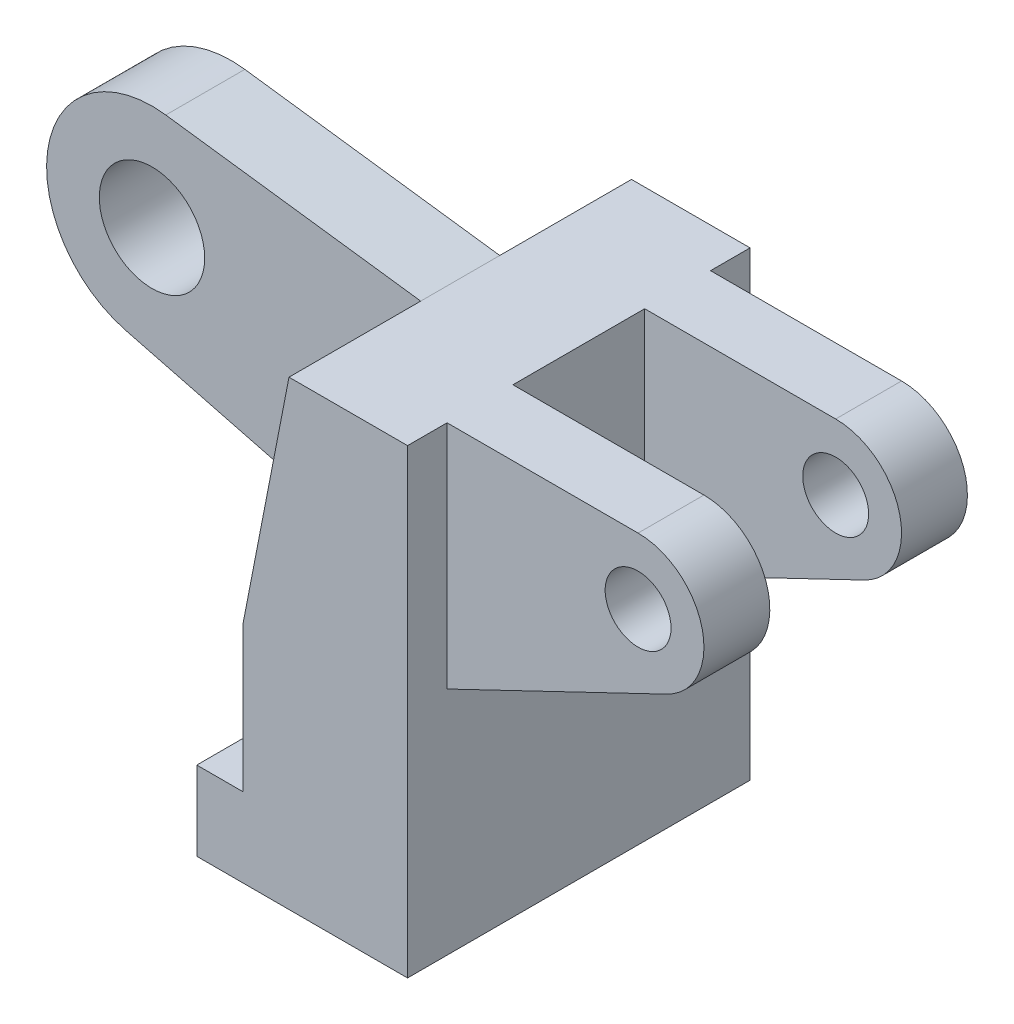
ISO-10303-21;
HEADER;
FILE_DESCRIPTION(('STEP AP214'),'2;1');
FILE_NAME('part.step','',(''),(''),'','','');
FILE_SCHEMA(('AUTOMOTIVE_DESIGN { 1 0 10303 214 1 1 1 1 }'));
ENDSEC;
DATA;
#1=APPLICATION_CONTEXT('core data for automotive mechanical design processes');
#2=APPLICATION_PROTOCOL_DEFINITION('international standard','automotive_design',2000,#1);
#3=PRODUCT_CONTEXT('',#1,'mechanical');
#4=PRODUCT('Part','Part','',(#3));
#5=PRODUCT_RELATED_PRODUCT_CATEGORY('part','',(#4));
#6=PRODUCT_DEFINITION_FORMATION('','',#4);
#7=PRODUCT_DEFINITION_CONTEXT('part definition',#1,'design');
#8=PRODUCT_DEFINITION('design','',#6,#7);
#9=PRODUCT_DEFINITION_SHAPE('','',#8);
#10=(LENGTH_UNIT() NAMED_UNIT(*) SI_UNIT(.MILLI.,.METRE.));
#11=(NAMED_UNIT(*) PLANE_ANGLE_UNIT() SI_UNIT($,.RADIAN.));
#12=(NAMED_UNIT(*) SI_UNIT($,.STERADIAN.) SOLID_ANGLE_UNIT());
#13=UNCERTAINTY_MEASURE_WITH_UNIT(LENGTH_MEASURE(1.E-05),#10,'distance_accuracy_value','');
#14=(GEOMETRIC_REPRESENTATION_CONTEXT(3) GLOBAL_UNCERTAINTY_ASSIGNED_CONTEXT((#13)) GLOBAL_UNIT_ASSIGNED_CONTEXT((#10,
#11,#12)) REPRESENTATION_CONTEXT('',''));
#15=CARTESIAN_POINT('',(0.,0.,0.));
#16=DIRECTION('',(0.,0.,1.));
#17=DIRECTION('',(1.,0.,0.));
#18=AXIS2_PLACEMENT_3D('',#15,#16,#17);
#19=CARTESIAN_POINT('',(7.,34.,0.));
#20=DIRECTION('',(-0.981615389668581,0.190869659102224,0.));
#21=DIRECTION('',(-0.190869659102224,-0.981615389668581,0.));
#22=AXIS2_PLACEMENT_3D('',#19,#20,#21);
#23=PLANE('',#22);
#24=DIRECTION('',(0.,0.,1.));
#25=VECTOR('',#24,1.);
#26=CARTESIAN_POINT('',(7.,34.,0.));
#27=LINE('',#26,#25);
#28=CARTESIAN_POINT('',(7.,34.,0.));
#29=VERTEX_POINT('',#28);
#30=CARTESIAN_POINT('',(7.,34.,20.));
#31=VERTEX_POINT('',#30);
#32=EDGE_CURVE('E206',#29,#31,#27,.T.);
#33=ORIENTED_EDGE('',*,*,#32,.T.);
#34=DIRECTION('',(-0.190869659102224,-0.981615389668581,0.));
#35=VECTOR('',#34,1.);
#36=CARTESIAN_POINT('',(0.374721189591083,-0.0728624535315993,20.));
#37=LINE('',#36,#35);
#38=CARTESIAN_POINT('',(14.,70.,20.));
#39=VERTEX_POINT('',#38);
#40=EDGE_CURVE('E543',#39,#31,#37,.T.);
#41=ORIENTED_EDGE('',*,*,#40,.F.);
#42=DIRECTION('',(0.,0.,1.));
#43=VECTOR('',#42,1.);
#44=CARTESIAN_POINT('',(14.,70.,0.));
#45=LINE('',#44,#43);
#46=CARTESIAN_POINT('',(14.,70.,0.));
#47=VERTEX_POINT('',#46);
#48=EDGE_CURVE('E210',#47,#39,#45,.T.);
#49=ORIENTED_EDGE('',*,*,#48,.F.);
#50=DIRECTION('',(-0.190869659102224,-0.981615389668581,0.));
#51=VECTOR('',#50,1.);
#52=CARTESIAN_POINT('',(7.,34.,0.));
#53=LINE('',#52,#51);
#54=EDGE_CURVE('E258',#47,#29,#53,.T.);
#55=ORIENTED_EDGE('',*,*,#54,.T.);
#56=EDGE_LOOP('',(#33,#41,#49,#55));
#57=FACE_BOUND('',#56,.T.);
#58=ADVANCED_FACE('F41',(#57),#23,.T.);
#59=CARTESIAN_POINT('',(0.,12.,52.));
#60=DIRECTION('',(0.,-1.,0.));
#61=DIRECTION('',(0.,0.,-1.));
#62=AXIS2_PLACEMENT_3D('',#59,#60,#61);
#63=PLANE('',#62);
#64=DIRECTION('',(0.,0.,1.));
#65=VECTOR('',#64,1.);
#66=CARTESIAN_POINT('',(7.,12.,0.));
#67=LINE('',#66,#65);
#68=CARTESIAN_POINT('',(7.,12.,0.));
#69=VERTEX_POINT('',#68);
#70=CARTESIAN_POINT('',(7.,12.,52.));
#71=VERTEX_POINT('',#70);
#72=EDGE_CURVE('E207',#69,#71,#67,.T.);
#73=ORIENTED_EDGE('',*,*,#72,.F.);
#74=DIRECTION('',(-1.,0.,0.));
#75=VECTOR('',#74,1.);
#76=CARTESIAN_POINT('',(0.,12.,0.));
#77=LINE('',#76,#75);
#78=CARTESIAN_POINT('',(0.,12.,0.));
#79=VERTEX_POINT('',#78);
#80=EDGE_CURVE('E224',#69,#79,#77,.T.);
#81=ORIENTED_EDGE('',*,*,#80,.T.);
#82=DIRECTION('',(0.,0.,-1.));
#83=VECTOR('',#82,1.);
#84=CARTESIAN_POINT('',(0.,12.,52.));
#85=LINE('',#84,#83);
#86=CARTESIAN_POINT('',(0.,12.,52.));
#87=VERTEX_POINT('',#86);
#88=EDGE_CURVE('E226',#87,#79,#85,.T.);
#89=ORIENTED_EDGE('',*,*,#88,.F.);
#90=DIRECTION('',(-1.,0.,0.));
#91=VECTOR('',#90,1.);
#92=CARTESIAN_POINT('',(0.,12.,52.));
#93=LINE('',#92,#91);
#94=EDGE_CURVE('E227',#71,#87,#93,.T.);
#95=ORIENTED_EDGE('',*,*,#94,.F.);
#96=EDGE_LOOP('',(#73,#81,#89,#95));
#97=FACE_BOUND('',#96,.T.);
#98=ADVANCED_FACE('F389',(#97),#63,.F.);
#99=CARTESIAN_POINT('',(0.,0.,52.));
#100=DIRECTION('',(1.,0.,0.));
#101=DIRECTION('',(0.,0.,-1.));
#102=AXIS2_PLACEMENT_3D('',#99,#100,#101);
#103=PLANE('',#102);
#104=DIRECTION('',(0.,-1.,0.));
#105=VECTOR('',#104,1.);
#106=CARTESIAN_POINT('',(0.,0.,0.));
#107=LINE('',#106,#105);
#108=CARTESIAN_POINT('',(0.,0.,0.));
#109=VERTEX_POINT('',#108);
#110=EDGE_CURVE('E232',#79,#109,#107,.T.);
#111=ORIENTED_EDGE('',*,*,#110,.T.);
#112=DIRECTION('',(0.,0.,-1.));
#113=VECTOR('',#112,1.);
#114=CARTESIAN_POINT('',(0.,0.,52.));
#115=LINE('',#114,#113);
#116=CARTESIAN_POINT('',(0.,0.,52.));
#117=VERTEX_POINT('',#116);
#118=EDGE_CURVE('E11',#117,#109,#115,.T.);
#119=ORIENTED_EDGE('',*,*,#118,.F.);
#120=DIRECTION('',(0.,-1.,0.));
#121=VECTOR('',#120,1.);
#122=CARTESIAN_POINT('',(0.,0.,52.));
#123=LINE('',#122,#121);
#124=EDGE_CURVE('E218',#87,#117,#123,.T.);
#125=ORIENTED_EDGE('',*,*,#124,.F.);
#126=ORIENTED_EDGE('',*,*,#88,.T.);
#127=EDGE_LOOP('',(#111,#119,#125,#126));
#128=FACE_BOUND('',#127,.T.);
#129=ADVANCED_FACE('F43',(#128),#103,.F.);
#130=CARTESIAN_POINT('',(0.,0.,52.));
#131=DIRECTION('',(0.,1.,0.));
#132=DIRECTION('',(0.,0.,1.));
#133=AXIS2_PLACEMENT_3D('',#130,#131,#132);
#134=PLANE('',#133);
#135=DIRECTION('',(1.,0.,0.));
#136=VECTOR('',#135,1.);
#137=CARTESIAN_POINT('',(0.,0.,0.));
#138=LINE('',#137,#136);
#139=CARTESIAN_POINT('',(32.,0.,0.));
#140=VERTEX_POINT('',#139);
#141=EDGE_CURVE('E231',#109,#140,#138,.T.);
#142=ORIENTED_EDGE('',*,*,#141,.T.);
#143=DIRECTION('',(0.,0.,-1.));
#144=VECTOR('',#143,1.);
#145=CARTESIAN_POINT('',(32.,0.,52.));
#146=LINE('',#145,#144);
#147=CARTESIAN_POINT('',(32.,0.,52.));
#148=VERTEX_POINT('',#147);
#149=EDGE_CURVE('E47',#148,#140,#146,.T.);
#150=ORIENTED_EDGE('',*,*,#149,.F.);
#151=DIRECTION('',(1.,0.,0.));
#152=VECTOR('',#151,1.);
#153=CARTESIAN_POINT('',(0.,0.,52.));
#154=LINE('',#153,#152);
#155=EDGE_CURVE('E225',#117,#148,#154,.T.);
#156=ORIENTED_EDGE('',*,*,#155,.F.);
#157=ORIENTED_EDGE('',*,*,#118,.T.);
#158=EDGE_LOOP('',(#142,#150,#156,#157));
#159=FACE_BOUND('',#158,.T.);
#160=ADVANCED_FACE('F426',(#159),#134,.F.);
#161=CARTESIAN_POINT('',(32.,12.,52.));
#162=DIRECTION('',(-1.,0.,0.));
#163=DIRECTION('',(0.,0.,1.));
#164=AXIS2_PLACEMENT_3D('',#161,#162,#163);
#165=PLANE('',#164);
#166=DIRECTION('',(0.,0.,1.));
#167=VECTOR('',#166,1.);
#168=CARTESIAN_POINT('',(32.,70.,0.));
#169=LINE('',#168,#167);
#170=CARTESIAN_POINT('',(32.,70.,16.));
#171=VERTEX_POINT('',#170);
#172=CARTESIAN_POINT('',(32.,70.,36.));
#173=VERTEX_POINT('',#172);
#174=EDGE_CURVE('E220',#171,#173,#169,.T.);
#175=ORIENTED_EDGE('',*,*,#174,.T.);
#176=DIRECTION('',(0.,-1.,0.));
#177=VECTOR('',#176,1.);
#178=CARTESIAN_POINT('',(32.,70.,36.));
#179=LINE('',#178,#177);
#180=CARTESIAN_POINT('',(32.,35.,36.));
#181=VERTEX_POINT('',#180);
#182=EDGE_CURVE('E65',#173,#181,#179,.T.);
#183=ORIENTED_EDGE('',*,*,#182,.T.);
#184=DIRECTION('',(0.,0.,1.));
#185=VECTOR('',#184,1.);
#186=CARTESIAN_POINT('',(32.,35.,36.));
#187=LINE('',#186,#185);
#188=CARTESIAN_POINT('',(32.,35.,46.));
#189=VERTEX_POINT('',#188);
#190=EDGE_CURVE('E301',#181,#189,#187,.T.);
#191=ORIENTED_EDGE('',*,*,#190,.T.);
#192=DIRECTION('',(0.,-1.,0.));
#193=VECTOR('',#192,1.);
#194=CARTESIAN_POINT('',(32.,70.,46.));
#195=LINE('',#194,#193);
#196=CARTESIAN_POINT('',(32.,70.,46.));
#197=VERTEX_POINT('',#196);
#198=EDGE_CURVE('E288',#197,#189,#195,.T.);
#199=ORIENTED_EDGE('',*,*,#198,.F.);
#200=CARTESIAN_POINT('',(32.,70.,52.));
#201=VERTEX_POINT('',#200);
#202=EDGE_CURVE('E217',#197,#201,#169,.T.);
#203=ORIENTED_EDGE('',*,*,#202,.T.);
#204=DIRECTION('',(0.,1.,0.));
#205=VECTOR('',#204,1.);
#206=CARTESIAN_POINT('',(32.,12.,52.));
#207=LINE('',#206,#205);
#208=EDGE_CURVE('E223',#148,#201,#207,.T.);
#209=ORIENTED_EDGE('',*,*,#208,.F.);
#210=ORIENTED_EDGE('',*,*,#149,.T.);
#211=DIRECTION('',(0.,1.,0.));
#212=VECTOR('',#211,1.);
#213=CARTESIAN_POINT('',(32.,12.,0.));
#214=LINE('',#213,#212);
#215=CARTESIAN_POINT('',(32.,70.,0.));
#216=VERTEX_POINT('',#215);
#217=EDGE_CURVE('E237',#140,#216,#214,.T.);
#218=ORIENTED_EDGE('',*,*,#217,.T.);
#219=CARTESIAN_POINT('',(32.,70.,6.));
#220=VERTEX_POINT('',#219);
#221=EDGE_CURVE('E214',#216,#220,#169,.T.);
#222=ORIENTED_EDGE('',*,*,#221,.T.);
#223=DIRECTION('',(0.,-1.,0.));
#224=VECTOR('',#223,1.);
#225=CARTESIAN_POINT('',(32.,70.,6.));
#226=LINE('',#225,#224);
#227=CARTESIAN_POINT('',(32.,35.,6.));
#228=VERTEX_POINT('',#227);
#229=EDGE_CURVE('E322',#220,#228,#226,.T.);
#230=ORIENTED_EDGE('',*,*,#229,.T.);
#231=DIRECTION('',(0.,0.,-1.));
#232=VECTOR('',#231,1.);
#233=CARTESIAN_POINT('',(32.,35.,16.));
#234=LINE('',#233,#232);
#235=CARTESIAN_POINT('',(32.,35.,16.));
#236=VERTEX_POINT('',#235);
#237=EDGE_CURVE('E263',#236,#228,#234,.T.);
#238=ORIENTED_EDGE('',*,*,#237,.F.);
#239=DIRECTION('',(0.,-1.,0.));
#240=VECTOR('',#239,1.);
#241=CARTESIAN_POINT('',(32.,70.,16.));
#242=LINE('',#241,#240);
#243=EDGE_CURVE('E330',#171,#236,#242,.T.);
#244=ORIENTED_EDGE('',*,*,#243,.F.);
#245=EDGE_LOOP('',(#175,#183,#191,#199,#203,#209,#210,#218,#222,#230,#238,#244));
#246=FACE_BOUND('',#245,.T.);
#247=ADVANCED_FACE('F245',(#246),#165,.F.);
#248=CARTESIAN_POINT('',(0.,0.,52.));
#249=DIRECTION('',(0.,0.,-1.));
#250=DIRECTION('',(-1.,0.,0.));
#251=AXIS2_PLACEMENT_3D('',#248,#249,#250);
#252=PLANE('',#251);
#253=ORIENTED_EDGE('',*,*,#124,.T.);
#254=ORIENTED_EDGE('',*,*,#155,.T.);
#255=ORIENTED_EDGE('',*,*,#208,.T.);
#256=DIRECTION('',(-1.,0.,0.));
#257=VECTOR('',#256,1.);
#258=CARTESIAN_POINT('',(32.,70.,52.));
#259=LINE('',#258,#257);
#260=CARTESIAN_POINT('',(14.,70.,52.));
#261=VERTEX_POINT('',#260);
#262=EDGE_CURVE('E268',#201,#261,#259,.T.);
#263=ORIENTED_EDGE('',*,*,#262,.T.);
#264=DIRECTION('',(-0.190869659102224,-0.981615389668581,0.));
#265=VECTOR('',#264,1.);
#266=CARTESIAN_POINT('',(7.,34.,52.));
#267=LINE('',#266,#265);
#268=CARTESIAN_POINT('',(7.,34.,52.));
#269=VERTEX_POINT('',#268);
#270=EDGE_CURVE('E261',#261,#269,#267,.T.);
#271=ORIENTED_EDGE('',*,*,#270,.T.);
#272=DIRECTION('',(0.,-1.,0.));
#273=VECTOR('',#272,1.);
#274=CARTESIAN_POINT('',(7.,12.,52.));
#275=LINE('',#274,#273);
#276=EDGE_CURVE('E202',#269,#71,#275,.T.);
#277=ORIENTED_EDGE('',*,*,#276,.T.);
#278=ORIENTED_EDGE('',*,*,#94,.T.);
#279=EDGE_LOOP('',(#253,#254,#255,#263,#271,#277,#278));
#280=FACE_BOUND('',#279,.T.);
#281=ADVANCED_FACE('F275',(#280),#252,.F.);
#282=CARTESIAN_POINT('',(0.,0.,0.));
#283=DIRECTION('',(0.,0.,-1.));
#284=DIRECTION('',(-1.,0.,0.));
#285=AXIS2_PLACEMENT_3D('',#282,#283,#284);
#286=PLANE('',#285);
#287=ORIENTED_EDGE('',*,*,#110,.F.);
#288=ORIENTED_EDGE('',*,*,#80,.F.);
#289=DIRECTION('',(0.,-1.,0.));
#290=VECTOR('',#289,1.);
#291=CARTESIAN_POINT('',(7.,12.,0.));
#292=LINE('',#291,#290);
#293=EDGE_CURVE('E259',#29,#69,#292,.T.);
#294=ORIENTED_EDGE('',*,*,#293,.F.);
#295=ORIENTED_EDGE('',*,*,#54,.F.);
#296=DIRECTION('',(-1.,0.,0.));
#297=VECTOR('',#296,1.);
#298=CARTESIAN_POINT('',(32.,70.,0.));
#299=LINE('',#298,#297);
#300=EDGE_CURVE('E251',#216,#47,#299,.T.);
#301=ORIENTED_EDGE('',*,*,#300,.F.);
#302=ORIENTED_EDGE('',*,*,#217,.F.);
#303=ORIENTED_EDGE('',*,*,#141,.F.);
#304=EDGE_LOOP('',(#287,#288,#294,#295,#301,#302,#303));
#305=FACE_BOUND('',#304,.T.);
#306=ADVANCED_FACE('F248',(#305),#286,.T.);
#307=CARTESIAN_POINT('',(7.,12.,0.));
#308=DIRECTION('',(-1.,0.,0.));
#309=DIRECTION('',(0.,0.,1.));
#310=AXIS2_PLACEMENT_3D('',#307,#308,#309);
#311=PLANE('',#310);
#312=ORIENTED_EDGE('',*,*,#276,.F.);
#313=CARTESIAN_POINT('',(7.,34.,32.));
#314=VERTEX_POINT('',#313);
#315=EDGE_CURVE('E193',#314,#269,#27,.T.);
#316=ORIENTED_EDGE('',*,*,#315,.F.);
#317=DIRECTION('',(0.,0.,-1.));
#318=VECTOR('',#317,1.);
#319=CARTESIAN_POINT('',(7.,34.,32.));
#320=LINE('',#319,#318);
#321=EDGE_CURVE('E175',#314,#31,#320,.T.);
#322=ORIENTED_EDGE('',*,*,#321,.T.);
#323=ORIENTED_EDGE('',*,*,#32,.F.);
#324=ORIENTED_EDGE('',*,*,#293,.T.);
#325=ORIENTED_EDGE('',*,*,#72,.T.);
#326=EDGE_LOOP('',(#312,#316,#322,#323,#324,#325));
#327=FACE_BOUND('',#326,.T.);
#328=ADVANCED_FACE('F205',(#327),#311,.T.);
#329=DIRECTION('',(-0.190869659102224,-0.981615389668581,0.));
#330=VECTOR('',#329,1.);
#331=CARTESIAN_POINT('',(0.374721189591083,-0.0728624535315993,32.));
#332=LINE('',#331,#330);
#333=CARTESIAN_POINT('',(14.,70.,32.));
#334=VERTEX_POINT('',#333);
#335=EDGE_CURVE('E57',#334,#314,#332,.T.);
#336=ORIENTED_EDGE('',*,*,#335,.T.);
#337=ORIENTED_EDGE('',*,*,#315,.T.);
#338=ORIENTED_EDGE('',*,*,#270,.F.);
#339=EDGE_CURVE('E197',#334,#261,#45,.T.);
#340=ORIENTED_EDGE('',*,*,#339,.F.);
#341=EDGE_LOOP('',(#336,#337,#338,#340));
#342=FACE_BOUND('',#341,.T.);
#343=ADVANCED_FACE('F194',(#342),#23,.T.);
#344=CARTESIAN_POINT('',(32.,70.,0.));
#345=DIRECTION('',(0.,1.,0.));
#346=DIRECTION('',(0.,0.,1.));
#347=AXIS2_PLACEMENT_3D('',#344,#345,#346);
#348=PLANE('',#347);
#349=ORIENTED_EDGE('',*,*,#262,.F.);
#350=ORIENTED_EDGE('',*,*,#202,.F.);
#351=DIRECTION('',(-1.,0.,0.));
#352=VECTOR('',#351,1.);
#353=CARTESIAN_POINT('',(32.,70.,46.));
#354=LINE('',#353,#352);
#355=CARTESIAN_POINT('',(61.,70.,46.));
#356=VERTEX_POINT('',#355);
#357=EDGE_CURVE('E307',#356,#197,#354,.T.);
#358=ORIENTED_EDGE('',*,*,#357,.F.);
#359=DIRECTION('',(0.,0.,1.));
#360=VECTOR('',#359,1.);
#361=CARTESIAN_POINT('',(61.,70.,36.));
#362=LINE('',#361,#360);
#363=CARTESIAN_POINT('',(61.,70.,36.));
#364=VERTEX_POINT('',#363);
#365=EDGE_CURVE('E318',#364,#356,#362,.T.);
#366=ORIENTED_EDGE('',*,*,#365,.F.);
#367=DIRECTION('',(-1.,0.,0.));
#368=VECTOR('',#367,1.);
#369=CARTESIAN_POINT('',(32.,70.,36.));
#370=LINE('',#369,#368);
#371=EDGE_CURVE('E294',#364,#173,#370,.T.);
#372=ORIENTED_EDGE('',*,*,#371,.T.);
#373=ORIENTED_EDGE('',*,*,#174,.F.);
#374=DIRECTION('',(-1.,0.,0.));
#375=VECTOR('',#374,1.);
#376=CARTESIAN_POINT('',(32.,70.,16.));
#377=LINE('',#376,#375);
#378=CARTESIAN_POINT('',(61.,70.,16.));
#379=VERTEX_POINT('',#378);
#380=EDGE_CURVE('E333',#379,#171,#377,.T.);
#381=ORIENTED_EDGE('',*,*,#380,.F.);
#382=DIRECTION('',(0.,0.,-1.));
#383=VECTOR('',#382,1.);
#384=CARTESIAN_POINT('',(61.,70.,16.));
#385=LINE('',#384,#383);
#386=CARTESIAN_POINT('',(61.,70.,6.));
#387=VERTEX_POINT('',#386);
#388=EDGE_CURVE('E337',#379,#387,#385,.T.);
#389=ORIENTED_EDGE('',*,*,#388,.T.);
#390=DIRECTION('',(-1.,0.,0.));
#391=VECTOR('',#390,1.);
#392=CARTESIAN_POINT('',(32.,70.,6.));
#393=LINE('',#392,#391);
#394=EDGE_CURVE('E332',#387,#220,#393,.T.);
#395=ORIENTED_EDGE('',*,*,#394,.T.);
#396=ORIENTED_EDGE('',*,*,#221,.F.);
#397=ORIENTED_EDGE('',*,*,#300,.T.);
#398=ORIENTED_EDGE('',*,*,#48,.T.);
#399=DIRECTION('',(0.,0.,-1.));
#400=VECTOR('',#399,1.);
#401=CARTESIAN_POINT('',(14.,70.,32.));
#402=LINE('',#401,#400);
#403=EDGE_CURVE('E184',#334,#39,#402,.T.);
#404=ORIENTED_EDGE('',*,*,#403,.F.);
#405=ORIENTED_EDGE('',*,*,#339,.T.);
#406=EDGE_LOOP('',(#349,#350,#358,#366,#372,#373,#381,#389,#395,#396,#397,#398,#404,#405));
#407=FACE_BOUND('',#406,.T.);
#408=ADVANCED_FACE('F273',(#407),#348,.T.);
#409=CARTESIAN_POINT('',(61.,60.,16.));
#410=DIRECTION('',(0.,0.,1.));
#411=DIRECTION('',(1.,0.,0.));
#412=AXIS2_PLACEMENT_3D('',#409,#410,#411);
#413=PLANE('',#412);
#414=ORIENTED_EDGE('',*,*,#243,.T.);
#415=DIRECTION('',(0.901653260251997,0.43245970711379,0.));
#416=VECTOR('',#415,1.);
#417=CARTESIAN_POINT('',(32.,35.,16.));
#418=LINE('',#417,#416);
#419=CARTESIAN_POINT('',(65.3245970711379,50.98346739748,16.));
#420=VERTEX_POINT('',#419);
#421=EDGE_CURVE('E329',#236,#420,#418,.T.);
#422=ORIENTED_EDGE('',*,*,#421,.T.);
#423=CARTESIAN_POINT('',(61.,60.,16.));
#424=DIRECTION('',(0.,0.,1.));
#425=DIRECTION('',(1.,0.,0.));
#426=AXIS2_PLACEMENT_3D('',#423,#424,#425);
#427=CIRCLE('',#426,10.);
#428=EDGE_CURVE('E334',#420,#379,#427,.T.);
#429=ORIENTED_EDGE('',*,*,#428,.T.);
#430=ORIENTED_EDGE('',*,*,#380,.T.);
#431=EDGE_LOOP('',(#414,#422,#429,#430));
#432=FACE_BOUND('',#431,.T.);
#433=CARTESIAN_POINT('',(61.,60.,16.));
#434=DIRECTION('',(0.,0.,1.));
#435=DIRECTION('',(1.,0.,0.));
#436=AXIS2_PLACEMENT_3D('',#433,#434,#435);
#437=CIRCLE('',#436,5.00000000000001);
#438=CARTESIAN_POINT('',(66.,60.,16.));
#439=VERTEX_POINT('',#438);
#440=EDGE_CURVE('E321',#439,#439,#437,.T.);
#441=ORIENTED_EDGE('',*,*,#440,.F.);
#442=EDGE_LOOP('',(#441));
#443=FACE_BOUND('',#442,.T.);
#444=ADVANCED_FACE('F366',(#432,#443),#413,.T.);
#445=CARTESIAN_POINT('',(61.,60.,6.));
#446=DIRECTION('',(0.,0.,1.));
#447=DIRECTION('',(1.,0.,0.));
#448=AXIS2_PLACEMENT_3D('',#445,#446,#447);
#449=PLANE('',#448);
#450=ORIENTED_EDGE('',*,*,#229,.F.);
#451=ORIENTED_EDGE('',*,*,#394,.F.);
#452=CARTESIAN_POINT('',(61.,60.,6.));
#453=DIRECTION('',(0.,0.,1.));
#454=DIRECTION('',(1.,0.,0.));
#455=AXIS2_PLACEMENT_3D('',#452,#453,#454);
#456=CIRCLE('',#455,10.);
#457=CARTESIAN_POINT('',(65.3245970711379,50.98346739748,6.));
#458=VERTEX_POINT('',#457);
#459=EDGE_CURVE('E345',#458,#387,#456,.T.);
#460=ORIENTED_EDGE('',*,*,#459,.F.);
#461=DIRECTION('',(0.901653260251997,0.43245970711379,0.));
#462=VECTOR('',#461,1.);
#463=CARTESIAN_POINT('',(32.,35.,6.));
#464=LINE('',#463,#462);
#465=EDGE_CURVE('E336',#228,#458,#464,.T.);
#466=ORIENTED_EDGE('',*,*,#465,.F.);
#467=EDGE_LOOP('',(#450,#451,#460,#466));
#468=FACE_BOUND('',#467,.T.);
#469=CARTESIAN_POINT('',(61.,60.,6.));
#470=DIRECTION('',(0.,0.,1.));
#471=DIRECTION('',(1.,0.,0.));
#472=AXIS2_PLACEMENT_3D('',#469,#470,#471);
#473=CIRCLE('',#472,5.00000000000001);
#474=CARTESIAN_POINT('',(66.,60.,6.));
#475=VERTEX_POINT('',#474);
#476=EDGE_CURVE('E319',#475,#475,#473,.T.);
#477=ORIENTED_EDGE('',*,*,#476,.T.);
#478=EDGE_LOOP('',(#477));
#479=FACE_BOUND('',#478,.T.);
#480=ADVANCED_FACE('F362',(#468,#479),#449,.F.);
#481=CARTESIAN_POINT('',(32.,35.,16.));
#482=DIRECTION('',(-0.43245970711379,0.901653260251997,0.));
#483=DIRECTION('',(-0.901653260251997,-0.43245970711379,0.));
#484=AXIS2_PLACEMENT_3D('',#481,#482,#483);
#485=PLANE('',#484);
#486=ORIENTED_EDGE('',*,*,#465,.T.);
#487=DIRECTION('',(0.,0.,-1.));
#488=VECTOR('',#487,1.);
#489=CARTESIAN_POINT('',(65.3245970711379,50.98346739748,16.));
#490=LINE('',#489,#488);
#491=EDGE_CURVE('E350',#420,#458,#490,.T.);
#492=ORIENTED_EDGE('',*,*,#491,.F.);
#493=ORIENTED_EDGE('',*,*,#421,.F.);
#494=ORIENTED_EDGE('',*,*,#237,.T.);
#495=EDGE_LOOP('',(#486,#492,#493,#494));
#496=FACE_BOUND('',#495,.T.);
#497=ADVANCED_FACE('F357',(#496),#485,.F.);
#498=CARTESIAN_POINT('',(61.,60.,16.));
#499=DIRECTION('',(0.,0.,-1.));
#500=DIRECTION('',(-1.,0.,0.));
#501=AXIS2_PLACEMENT_3D('',#498,#499,#500);
#502=CYLINDRICAL_SURFACE('',#501,10.);
#503=ORIENTED_EDGE('',*,*,#459,.T.);
#504=ORIENTED_EDGE('',*,*,#388,.F.);
#505=ORIENTED_EDGE('',*,*,#428,.F.);
#506=ORIENTED_EDGE('',*,*,#491,.T.);
#507=EDGE_LOOP('',(#503,#504,#505,#506));
#508=FACE_BOUND('',#507,.T.);
#509=ADVANCED_FACE('F364',(#508),#502,.T.);
#510=CARTESIAN_POINT('',(61.,60.,16.));
#511=DIRECTION('',(0.,0.,-1.));
#512=DIRECTION('',(-1.,0.,0.));
#513=AXIS2_PLACEMENT_3D('',#510,#511,#512);
#514=CYLINDRICAL_SURFACE('',#513,5.00000000000001);
#515=ORIENTED_EDGE('',*,*,#440,.T.);
#516=EDGE_LOOP('',(#515));
#517=FACE_BOUND('',#516,.T.);
#518=ORIENTED_EDGE('',*,*,#476,.F.);
#519=EDGE_LOOP('',(#518));
#520=FACE_BOUND('',#519,.T.);
#521=ADVANCED_FACE('F372',(#517,#520),#514,.F.);
#522=CARTESIAN_POINT('',(61.,60.,36.));
#523=DIRECTION('',(0.,0.,1.));
#524=DIRECTION('',(1.,0.,0.));
#525=AXIS2_PLACEMENT_3D('',#522,#523,#524);
#526=CYLINDRICAL_SURFACE('',#525,10.);
#527=CARTESIAN_POINT('',(61.,60.,46.));
#528=DIRECTION('',(0.,0.,1.));
#529=DIRECTION('',(1.,0.,0.));
#530=AXIS2_PLACEMENT_3D('',#527,#528,#529);
#531=CIRCLE('',#530,10.);
#532=CARTESIAN_POINT('',(65.3245970711379,50.98346739748,46.));
#533=VERTEX_POINT('',#532);
#534=EDGE_CURVE('E309',#533,#356,#531,.T.);
#535=ORIENTED_EDGE('',*,*,#534,.F.);
#536=DIRECTION('',(0.,0.,1.));
#537=VECTOR('',#536,1.);
#538=CARTESIAN_POINT('',(65.3245970711379,50.98346739748,36.));
#539=LINE('',#538,#537);
#540=CARTESIAN_POINT('',(65.3245970711379,50.98346739748,36.));
#541=VERTEX_POINT('',#540);
#542=EDGE_CURVE('E316',#541,#533,#539,.T.);
#543=ORIENTED_EDGE('',*,*,#542,.F.);
#544=CARTESIAN_POINT('',(61.,60.,36.));
#545=DIRECTION('',(0.,0.,1.));
#546=DIRECTION('',(1.,0.,0.));
#547=AXIS2_PLACEMENT_3D('',#544,#545,#546);
#548=CIRCLE('',#547,10.);
#549=EDGE_CURVE('E297',#541,#364,#548,.T.);
#550=ORIENTED_EDGE('',*,*,#549,.T.);
#551=ORIENTED_EDGE('',*,*,#365,.T.);
#552=EDGE_LOOP('',(#535,#543,#550,#551));
#553=FACE_BOUND('',#552,.T.);
#554=ADVANCED_FACE('F380',(#553),#526,.T.);
#555=CARTESIAN_POINT('',(32.,35.,36.));
#556=DIRECTION('',(0.43245970711379,-0.901653260251997,0.));
#557=DIRECTION('',(0.901653260251997,0.43245970711379,0.));
#558=AXIS2_PLACEMENT_3D('',#555,#556,#557);
#559=PLANE('',#558);
#560=DIRECTION('',(0.901653260251997,0.43245970711379,0.));
#561=VECTOR('',#560,1.);
#562=CARTESIAN_POINT('',(32.,35.,46.));
#563=LINE('',#562,#561);
#564=EDGE_CURVE('E293',#189,#533,#563,.T.);
#565=ORIENTED_EDGE('',*,*,#564,.F.);
#566=ORIENTED_EDGE('',*,*,#190,.F.);
#567=DIRECTION('',(0.901653260251997,0.43245970711379,0.));
#568=VECTOR('',#567,1.);
#569=CARTESIAN_POINT('',(32.,35.,36.));
#570=LINE('',#569,#568);
#571=EDGE_CURVE('E302',#181,#541,#570,.T.);
#572=ORIENTED_EDGE('',*,*,#571,.T.);
#573=ORIENTED_EDGE('',*,*,#542,.T.);
#574=EDGE_LOOP('',(#565,#566,#572,#573));
#575=FACE_BOUND('',#574,.T.);
#576=ADVANCED_FACE('F436',(#575),#559,.T.);
#577=CARTESIAN_POINT('',(61.,60.,36.));
#578=DIRECTION('',(0.,0.,-1.));
#579=DIRECTION('',(1.,0.,0.));
#580=AXIS2_PLACEMENT_3D('',#577,#578,#579);
#581=PLANE('',#580);
#582=CARTESIAN_POINT('',(61.,60.,36.));
#583=DIRECTION('',(0.,0.,1.));
#584=DIRECTION('',(1.,0.,0.));
#585=AXIS2_PLACEMENT_3D('',#582,#583,#584);
#586=CIRCLE('',#585,5.00000000000001);
#587=CARTESIAN_POINT('',(66.,60.,36.));
#588=VERTEX_POINT('',#587);
#589=EDGE_CURVE('E290',#588,#588,#586,.T.);
#590=ORIENTED_EDGE('',*,*,#589,.T.);
#591=EDGE_LOOP('',(#590));
#592=FACE_BOUND('',#591,.T.);
#593=ORIENTED_EDGE('',*,*,#182,.F.);
#594=ORIENTED_EDGE('',*,*,#371,.F.);
#595=ORIENTED_EDGE('',*,*,#549,.F.);
#596=ORIENTED_EDGE('',*,*,#571,.F.);
#597=EDGE_LOOP('',(#593,#594,#595,#596));
#598=FACE_BOUND('',#597,.T.);
#599=ADVANCED_FACE('F443',(#592,#598),#581,.T.);
#600=CARTESIAN_POINT('',(61.,60.,46.));
#601=DIRECTION('',(0.,0.,-1.));
#602=DIRECTION('',(1.,0.,0.));
#603=AXIS2_PLACEMENT_3D('',#600,#601,#602);
#604=PLANE('',#603);
#605=CARTESIAN_POINT('',(61.,60.,46.));
#606=DIRECTION('',(0.,0.,1.));
#607=DIRECTION('',(1.,0.,0.));
#608=AXIS2_PLACEMENT_3D('',#605,#606,#607);
#609=CIRCLE('',#608,5.00000000000001);
#610=CARTESIAN_POINT('',(66.,60.,46.));
#611=VERTEX_POINT('',#610);
#612=EDGE_CURVE('E181',#611,#611,#609,.T.);
#613=ORIENTED_EDGE('',*,*,#612,.F.);
#614=EDGE_LOOP('',(#613));
#615=FACE_BOUND('',#614,.T.);
#616=ORIENTED_EDGE('',*,*,#198,.T.);
#617=ORIENTED_EDGE('',*,*,#564,.T.);
#618=ORIENTED_EDGE('',*,*,#534,.T.);
#619=ORIENTED_EDGE('',*,*,#357,.T.);
#620=EDGE_LOOP('',(#616,#617,#618,#619));
#621=FACE_BOUND('',#620,.T.);
#622=ADVANCED_FACE('F451',(#615,#621),#604,.F.);
#623=CARTESIAN_POINT('',(61.,60.,36.));
#624=DIRECTION('',(0.,0.,1.));
#625=DIRECTION('',(1.,0.,0.));
#626=AXIS2_PLACEMENT_3D('',#623,#624,#625);
#627=CYLINDRICAL_SURFACE('',#626,5.00000000000001);
#628=ORIENTED_EDGE('',*,*,#589,.F.);
#629=EDGE_LOOP('',(#628));
#630=FACE_BOUND('',#629,.T.);
#631=ORIENTED_EDGE('',*,*,#612,.T.);
#632=EDGE_LOOP('',(#631));
#633=FACE_BOUND('',#632,.T.);
#634=ADVANCED_FACE('F464',(#630,#633),#627,.F.);
#635=CARTESIAN_POINT('',(8.66827838339267,33.5692153873307,32.));
#636=DIRECTION('',(-0.250020124525285,-0.968240640198686,0.));
#637=DIRECTION('',(0.968240640198686,-0.250020124525286,0.));
#638=AXIS2_PLACEMENT_3D('',#635,#636,#637);
#639=PLANE('',#638);
#640=DIRECTION('',(-0.968240640198686,0.250020124525285,0.));
#641=VECTOR('',#640,1.);
#642=CARTESIAN_POINT('',(8.66827838339267,33.5692153873307,20.));
#643=LINE('',#642,#641);
#644=CARTESIAN_POINT('',(-30.8017067998107,43.7611968027056,20.));
#645=VERTEX_POINT('',#644);
#646=EDGE_CURVE('E179',#31,#645,#643,.T.);
#647=ORIENTED_EDGE('',*,*,#646,.F.);
#648=ORIENTED_EDGE('',*,*,#321,.F.);
#649=DIRECTION('',(-0.968240640198686,0.250020124525285,0.));
#650=VECTOR('',#649,1.);
#651=CARTESIAN_POINT('',(8.66827838339267,33.5692153873307,32.));
#652=LINE('',#651,#650);
#653=CARTESIAN_POINT('',(-30.8017067998107,43.7611968027056,32.));
#654=VERTEX_POINT('',#653);
#655=EDGE_CURVE('E177',#314,#654,#652,.T.);
#656=ORIENTED_EDGE('',*,*,#655,.T.);
#657=DIRECTION('',(0.,0.,-1.));
#658=VECTOR('',#657,1.);
#659=CARTESIAN_POINT('',(-30.8017067998107,43.7611968027056,32.));
#660=LINE('',#659,#658);
#661=EDGE_CURVE('E282',#654,#645,#660,.T.);
#662=ORIENTED_EDGE('',*,*,#661,.T.);
#663=EDGE_LOOP('',(#647,#648,#656,#662));
#664=FACE_BOUND('',#663,.T.);
#665=ADVANCED_FACE('F171',(#664),#639,.T.);
#666=CARTESIAN_POINT('',(9.33246904056323,70.6168441636091,32.));
#667=DIRECTION('',(-0.131017239685582,-0.991380090028628,0.));
#668=DIRECTION('',(0.991380090028628,-0.131017239685582,0.));
#669=AXIS2_PLACEMENT_3D('',#666,#667,#668);
#670=PLANE('',#669);
#671=DIRECTION('',(-0.991380090028628,0.131017239685582,0.));
#672=VECTOR('',#671,1.);
#673=CARTESIAN_POINT('',(9.33246904056323,70.6168441636091,20.));
#674=LINE('',#673,#672);
#675=CARTESIAN_POINT('',(-24.7051089724368,75.1151284863426,20.));
#676=VERTEX_POINT('',#675);
#677=EDGE_CURVE('E544',#39,#676,#674,.T.);
#678=ORIENTED_EDGE('',*,*,#677,.T.);
#679=DIRECTION('',(0.,0.,-1.));
#680=VECTOR('',#679,1.);
#681=CARTESIAN_POINT('',(-24.7051089724368,75.1151284863426,32.));
#682=LINE('',#681,#680);
#683=CARTESIAN_POINT('',(-24.7051089724368,75.1151284863426,32.));
#684=VERTEX_POINT('',#683);
#685=EDGE_CURVE('E278',#684,#676,#682,.T.);
#686=ORIENTED_EDGE('',*,*,#685,.F.);
#687=DIRECTION('',(-0.991380090028628,0.131017239685582,0.));
#688=VECTOR('',#687,1.);
#689=CARTESIAN_POINT('',(9.33246904056323,70.6168441636091,32.));
#690=LINE('',#689,#688);
#691=EDGE_CURVE('E200',#334,#684,#690,.T.);
#692=ORIENTED_EDGE('',*,*,#691,.F.);
#693=ORIENTED_EDGE('',*,*,#403,.T.);
#694=EDGE_LOOP('',(#678,#686,#692,#693));
#695=FACE_BOUND('',#694,.T.);
#696=ADVANCED_FACE('F486',(#695),#670,.F.);
#697=CARTESIAN_POINT('',(-26.8013848074061,59.2530470458845,32.));
#698=DIRECTION('',(0.,0.,-1.));
#699=DIRECTION('',(-1.,0.,0.));
#700=AXIS2_PLACEMENT_3D('',#697,#698,#699);
#701=CYLINDRICAL_SURFACE('',#700,8.);
#702=CARTESIAN_POINT('',(-26.8013848074061,59.2530470458845,32.));
#703=DIRECTION('',(0.,0.,1.));
#704=DIRECTION('',(1.,0.,0.));
#705=AXIS2_PLACEMENT_3D('',#702,#703,#704);
#706=CIRCLE('',#705,8.);
#707=CARTESIAN_POINT('',(-18.8013848074061,59.2530470458845,32.));
#708=VERTEX_POINT('',#707);
#709=EDGE_CURVE('E190',#708,#708,#706,.T.);
#710=ORIENTED_EDGE('',*,*,#709,.T.);
#711=EDGE_LOOP('',(#710));
#712=FACE_BOUND('',#711,.T.);
#713=CARTESIAN_POINT('',(-26.8013848074061,59.2530470458845,20.));
#714=DIRECTION('',(0.,0.,1.));
#715=DIRECTION('',(1.,0.,0.));
#716=AXIS2_PLACEMENT_3D('',#713,#714,#715);
#717=CIRCLE('',#716,8.);
#718=CARTESIAN_POINT('',(-18.8013848074061,59.2530470458845,20.));
#719=VERTEX_POINT('',#718);
#720=EDGE_CURVE('E537',#719,#719,#717,.T.);
#721=ORIENTED_EDGE('',*,*,#720,.F.);
#722=EDGE_LOOP('',(#721));
#723=FACE_BOUND('',#722,.T.);
#724=ADVANCED_FACE('F494',(#712,#723),#701,.F.);
#725=CARTESIAN_POINT('',(-26.8013848074061,59.2530470458845,32.));
#726=DIRECTION('',(0.,0.,-1.));
#727=DIRECTION('',(-1.,0.,0.));
#728=AXIS2_PLACEMENT_3D('',#725,#726,#727);
#729=CYLINDRICAL_SURFACE('',#728,16.);
#730=CARTESIAN_POINT('',(-26.8013848074061,59.2530470458845,20.));
#731=DIRECTION('',(0.,0.,1.));
#732=DIRECTION('',(1.,0.,0.));
#733=AXIS2_PLACEMENT_3D('',#730,#731,#732);
#734=CIRCLE('',#733,16.);
#735=EDGE_CURVE('E541',#676,#645,#734,.T.);
#736=ORIENTED_EDGE('',*,*,#735,.T.);
#737=ORIENTED_EDGE('',*,*,#661,.F.);
#738=CARTESIAN_POINT('',(-26.8013848074061,59.2530470458845,32.));
#739=DIRECTION('',(0.,0.,1.));
#740=DIRECTION('',(1.,0.,0.));
#741=AXIS2_PLACEMENT_3D('',#738,#739,#740);
#742=CIRCLE('',#741,16.);
#743=EDGE_CURVE('E189',#684,#654,#742,.T.);
#744=ORIENTED_EDGE('',*,*,#743,.F.);
#745=ORIENTED_EDGE('',*,*,#685,.T.);
#746=EDGE_LOOP('',(#736,#737,#744,#745));
#747=FACE_BOUND('',#746,.T.);
#748=ADVANCED_FACE('F505',(#747),#729,.T.);
#749=CARTESIAN_POINT('',(0.,0.,32.));
#750=DIRECTION('',(0.,0.,1.));
#751=DIRECTION('',(1.,0.,0.));
#752=AXIS2_PLACEMENT_3D('',#749,#750,#751);
#753=PLANE('',#752);
#754=ORIENTED_EDGE('',*,*,#709,.F.);
#755=EDGE_LOOP('',(#754));
#756=FACE_BOUND('',#755,.T.);
#757=ORIENTED_EDGE('',*,*,#655,.F.);
#758=ORIENTED_EDGE('',*,*,#335,.F.);
#759=ORIENTED_EDGE('',*,*,#691,.T.);
#760=ORIENTED_EDGE('',*,*,#743,.T.);
#761=EDGE_LOOP('',(#757,#758,#759,#760));
#762=FACE_BOUND('',#761,.T.);
#763=ADVANCED_FACE('F188',(#756,#762),#753,.T.);
#764=CARTESIAN_POINT('',(0.,0.,20.));
#765=DIRECTION('',(0.,0.,1.));
#766=DIRECTION('',(1.,0.,0.));
#767=AXIS2_PLACEMENT_3D('',#764,#765,#766);
#768=PLANE('',#767);
#769=ORIENTED_EDGE('',*,*,#720,.T.);
#770=EDGE_LOOP('',(#769));
#771=FACE_BOUND('',#770,.T.);
#772=ORIENTED_EDGE('',*,*,#646,.T.);
#773=ORIENTED_EDGE('',*,*,#735,.F.);
#774=ORIENTED_EDGE('',*,*,#677,.F.);
#775=ORIENTED_EDGE('',*,*,#40,.T.);
#776=EDGE_LOOP('',(#772,#773,#774,#775));
#777=FACE_BOUND('',#776,.T.);
#778=ADVANCED_FACE('F524',(#771,#777),#768,.F.);
#779=CLOSED_SHELL('',(#58,#98,#129,#160,#247,#281,#306,#328,#343,#408,#444,#480,#497,#509,#521,
#554,#576,#599,#622,#634,#665,#696,#724,#748,#763,#778));
#780=MANIFOLD_SOLID_BREP('B2',#779);
#781=ADVANCED_BREP_SHAPE_REPRESENTATION('',(#18,#780),#14);
#782=SHAPE_DEFINITION_REPRESENTATION(#9,#781);
ENDSEC;
END-ISO-10303-21;
